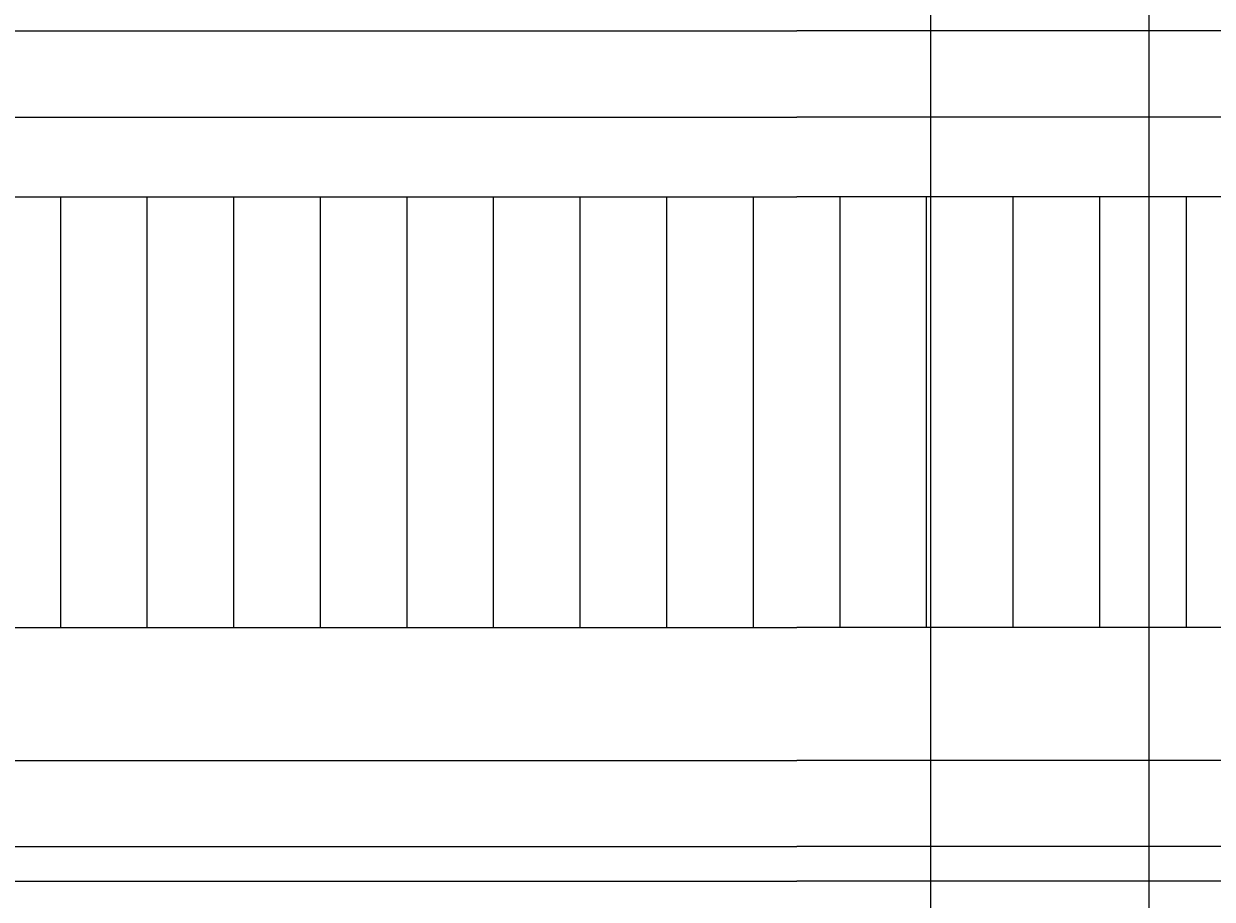
# Model space of a CAD drawing. Units: millimetres. Extents: x 2332 to 5836, y -853 to 2199.
# Tile 9 of 16: x 3986 to 4331, y 753 to 1007. Entities that reach past the tile are written whole.
import ezdxf

# ---------------------------------------------------------------- set-up
doc = ezdxf.new("R2010")
doc.units = ezdxf.units.MM
for name, color, linetype, lineweight in [('A-ANNO-DIMS', 2, 'Continuous', 18), ('A-EQPM', 7, 'Continuous', 25), ('A-EQPM-PATT', 7, 'Continuous', 13)]:
    doc.layers.add(name, color=color, linetype=linetype, lineweight=lineweight)
doc.styles.get("Standard").update_dxf_attribs({"font": 'arial.ttf'})
doc.dimstyles.new('ISO-25', dxfattribs={"dimtxt": 2.5, "dimasz": 2.5, "dimexe": 1.25, "dimexo": 0.625, "dimtad": 1, "dimtxsty": 'Standard', "dimcen": 2.5, "dimadec": 0, "dimazin": 0, "dimtfac": 1, "dimtmove": 0, "dimatfit": 3, "dimfxl": 1, "dimarcsym": 0})

# ---------------------------------------------------------------- blocks, each defined once
blk = doc.blocks.new('*D27')
at = {"layer": 'A-ANNO-DIMS', "color": 0, "lineweight": -2, "transparency": 16777216}
for p, q in [((3772.66, 830.99), (3772.66, -853.1)), ((4647.42, 830.99), (4647.42, -853.1)), ((3775.16, -851.85), (4644.92, -851.85))]:
    blk.add_line(p, q, dxfattribs=at)
at = {"layer": 'A-ANNO-DIMS', "color": 0, "transparency": 16777216}
for points in [[(3775.16, -851.43), (3775.16, -852.26), (3772.66, -851.85)], [(4644.92, -851.43), (4644.92, -852.26), (4647.42, -851.85)]]:
    blk.add_solid(points, dxfattribs=at)
at = {"layer": 'Defpoints', "color": 0, "transparency": 16777216}
for p in [(3772.66, 831.62), (4647.42, 831.62), (4647.42, -851.85)]:
    blk.add_point(p, dxfattribs=at)
at = {"layer": 'A-ANNO-DIMS', "color": 0, "transparency": 16777216, "insert": (4210.04, -849.95), "char_height": 2.5, "attachment_point": 5}
blk.add_mtext('874.8', dxfattribs=at)
blk = doc.blocks.new('*D33')
at = {"layer": 'A-ANNO-DIMS', "color": 0, "lineweight": -2, "transparency": 16777216}
for p, q in [((4248.92, 1016.42), (4248.92, -853.1)), ((4312.24, 1016.42), (4312.24, -853.1)), ((4251.42, -851.85), (4309.74, -851.85))]:
    blk.add_line(p, q, dxfattribs=at)
at = {"layer": 'A-ANNO-DIMS', "color": 0, "transparency": 16777216}
for points in [[(4251.42, -851.43), (4251.42, -852.26), (4248.92, -851.85)], [(4309.74, -851.43), (4309.74, -852.26), (4312.24, -851.85)]]:
    blk.add_solid(points, dxfattribs=at)
at = {"layer": 'Defpoints', "color": 0, "transparency": 16777216}
for p in [(4248.92, 1017.04), (4312.24, 1017.04), (4312.24, -851.85)]:
    blk.add_point(p, dxfattribs=at)
at = {"layer": 'A-ANNO-DIMS', "color": 0, "transparency": 16777216, "insert": (4280.58, -849.94), "char_height": 2.5, "attachment_point": 5}
blk.add_mtext('63.33', dxfattribs=at)

msp = doc.modelspace()

# ---------------------------------------------------------------- hatches: boundary and pattern name
at = {"layer": 'A-EQPM-PATT'}
h = msp.add_hatch(dxfattribs=at)
h.set_pattern_fill('ANSI31', color=256, scale=7.9164, angle=45, style=0)
h.paths.add_polyline_path([(3772.661, 831.62), (4647.419, 831.62), (4647.419, 956.62), (3772.661, 956.62)])

# ---------------------------------------------------------------- linework, layer by layer
at = {"layer": 'A-EQPM'}
for p, q in [((3646.468, 1004.801), (4210.04, 1004.801)), ((4773.612, 1004.801), (4210.04, 1004.801)), ((3679.541, 979.768), (4210.04, 979.768)), ((4740.539, 979.768), (4210.04, 979.768)), ((3772.661, 956.62), (4210.04, 956.62)), ((4647.419, 956.62), (4210.04, 956.62)), ((3772.661, 831.62), (4210.04, 831.62)), ((4647.419, 831.62), (4210.04, 831.62)), ((3679.541, 793.058), (4210.04, 793.058)), ((4740.539, 793.058), (4210.04, 793.058)), ((3679.541, 768.058), (4210.04, 768.058)), ((4740.539, 768.058), (4210.04, 768.058)), ((3679.541, 758.058), (4210.04, 758.058)), ((4740.539, 758.058), (4210.04, 758.058))]:
    msp.add_line(p, q, dxfattribs=at)

# ---------------------------------------------------------------- dimensions: what is measured, and where the dimension line sits
at = {"layer": 'A-ANNO-DIMS'}
for base, p1, p2, override, picture, middle in [((4312.243, -851.847), (4248.917, 1017.045), (4312.243, 1017.045), {"dimdec": 2, "dimlfac": 1, "dimrnd": 0, "dimzin": 0, "dimdsep": 46, "dimlunit": 2}, '*D33', (4280.58, -849.944)), ((4647.419, -851.847), (3772.661, 831.62), (4647.419, 831.62), {"dimdec": 1, "dimlfac": 1, "dimrnd": 0, "dimzin": 0, "dimdsep": 46, "dimlunit": 2}, '*D27', (4210.04, -849.945))]:
    dim = msp.add_linear_dim(base=base, p1=p1, p2=p2, dimstyle='ISO-25', override=override, dxfattribs=at)
    dim.commit()
    dim.dimension.update_dxf_attribs({"geometry": picture, "text_midpoint": middle})

doc.saveas('drawing.dxf')
